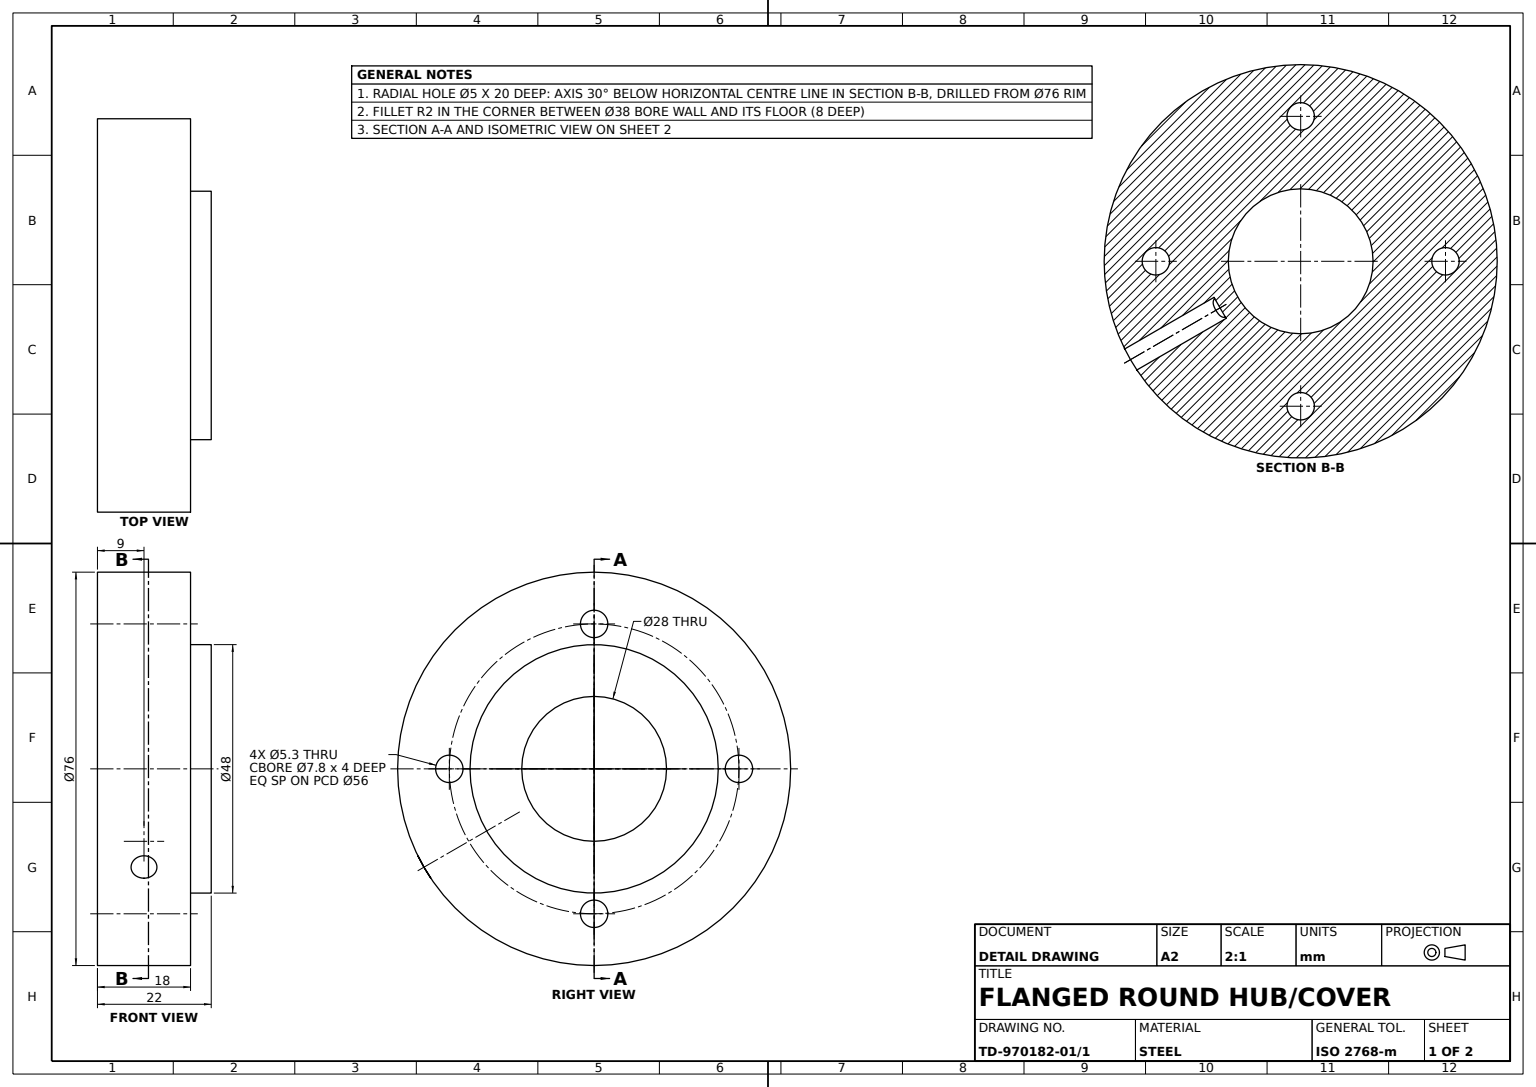
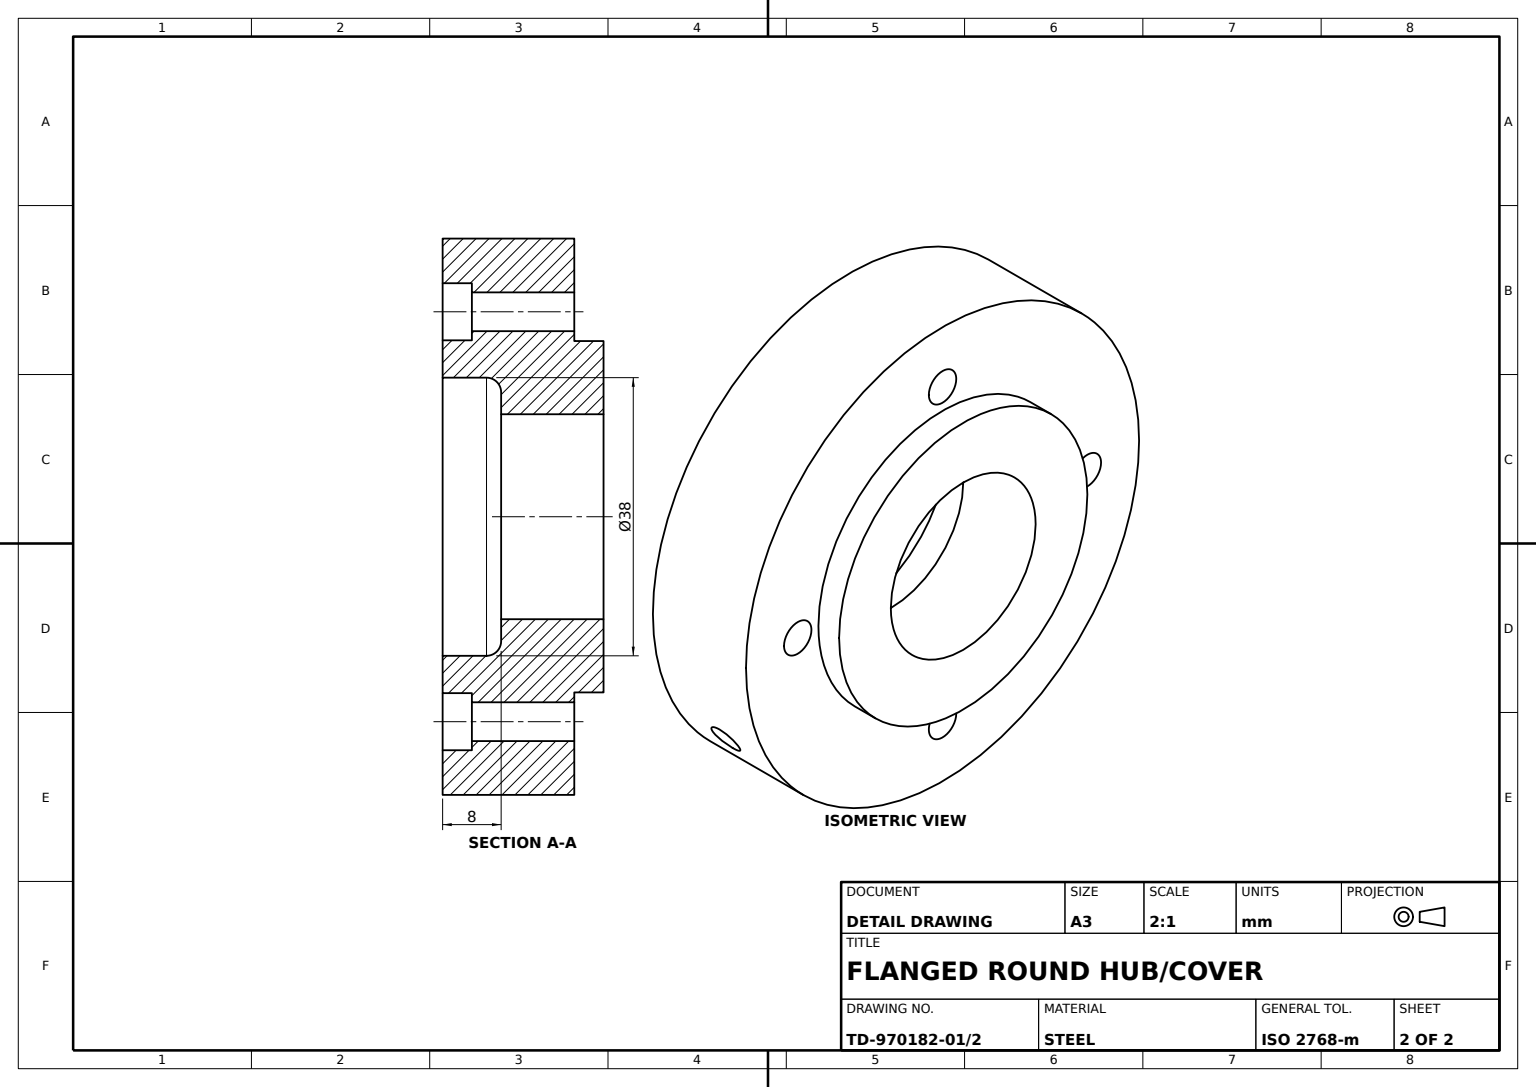
SolidWorks part; units mm, degrees
material "Plain Carbon Steel"
ref_plane "Front Plane" through (0, 0, 0) normal (0, 0, 1) x (1, 0, 0)
ref_plane "Top Plane" through (0, 0, 0) normal (0, 1, 0) x (1, 0, 0)
ref_plane "Right Plane" through (0, 0, 0) normal (1, 0, 0) x (0, 0, -1)
sketch "Base Disc Sketch" plane through (0, 0, 0) normal (0, 1, 0) x (1, 0, 0)
  line L0 (0, 77.9975) -> (0, -76.7867) construction
  line L1 (115.0286, 0) -> (-119.4683, 0) construction
  circle A0 centre (0, 0) radius 38
  dimension "D1" = 76
extrude "Base Disc Ø76x18" add sketch "Base Disc Sketch" along normal mid plane 18 contours A0
sketch "Spigot Sketch" plane through (0, 9, 0) normal (0, 1, 0) x (1, 0, 0)
  circle A0 centre (0, 0) radius 24
  dimension "D1" = 48
extrude "Spigot Ø48x8" add sketch "Spigot Sketch" along normal mid plane 8 contours A0
sketch "Mounting Hole Positions PCD Ø56" plane through (0, -9, 0) normal (0, -1, 0) x (1, 0, 0)
  line L0 (0, 41.7054) -> (0, -43.0294) construction
  line L1 (48.7836, 0) -> (-51.8389, 0) construction
  circle A0 centre (0, 0) radius 28 construction
  dimension "D1" = 56
hole_wizard "Counterbored Mounting Holes Ø5.3" positions "3DSketch1" profile "Sketch4" legacy
sketch3d "3DSketch1"
  line L0 (0, -9, 41.7054) -> (0, -9, -43.0294) construction
  line L1 (48.7836, -9, 0) -> (-51.8389, -9, 0) construction
  circle A0 centre (0, -9, 0) radius 28 construction
  point P0 (0, -9, 28)
  point P6 (0, -37, 0)
  point P7 (28, -9, 0)
  point P11 (0, -9, -28)
  point P13 (-28, -9, 0)
sketch "Sketch4" plane through (0, -9, 28) normal (1, 0, 0) x (0, 0, -1)
  line L0 (0, 0) -> (0, 18)
  line L1 (0, 18) -> (2.65, 18)
  line L2 (2.65, 18) -> (2.65, 4)
  line L3 (2.65, 4) -> (3.9, 4)
  line L4 (3.9, 4) -> (3.9, 0)
  line L5 (3.9, 0) -> (0, 0)
  line L6 (0, 110) -> (0, -10) construction
  dimension "Diameter" = 5.3
  dimension "Depth" = 18
  dimension "C-Bore Diameter" = 7.8
  dimension "C-Bore Depth" = 4
sketch "Counterbore Bore Sketch" plane through (0, -9, 0) normal (0, -1, 0) x (1, 0, 0)
  circle A0 centre (0, 0) radius 19
  dimension "D1" = 38
extrude "Counterbore Bore Ø38x16" cut sketch "Counterbore Bore Sketch" against normal mid plane 16 contours A0
sketch "Through Bore Sketch" plane through (0, -1, 0) normal (0, -1, 0) x (1, 0, 0)
  circle A0 centre (0, 0) radius 14
  dimension "D1" = 28
extrude "Through Bore Ø28" cut sketch "Through Bore Sketch" against normal up to next
fillet "Bore Edge Fillet R2" radius 2 1 edges at (0, -1, -19)
sketch "Radial Hole Plane Sketch 30deg" plane through (0, 0, 0) normal (0, 1, 0) x (1, 0, 0)
  line L0 (0, 46.1966) -> (0, -42.5625) construction
  line L1 (0, 0) -> (19.7257, -34.166) construction
  circle A0 centre (0, 0) radius 38 construction
  arc A1 (0, -38) -> (0, 38) centre (0, 0) ccw
  dimension "D1" = 30
ref_plane "Radial Hole Plane" through (19, 0, 32.909) normal (0.5, 0, 0.866) x (0.866, 0, -0.5)
hole_wizard "Radial Hole Ø5x20" positions "Sketch17" profile "Sketch18" legacy
sketch "Sketch17" plane through (19, 0, 32.909) normal (0.5, 0, 0.866) x (0.866, 0, -0.5)
  point P0 (0, 0)
sketch "Sketch18" plane through (19, 0, 32.909) normal (0, 1, 0) x (0.866, 0, -0.5)
  line L0 (0, 0) -> (0, 20)
  line L1 (0, 20) -> (2.5, 20)
  line L2 (2.5, 20) -> (2.5, 0)
  line L3 (2.5, 0) -> (0, 0)
  line L4 (0, 110) -> (0, -10) construction
  dimension "Diameter" = 5
  dimension "Depth" = 20
